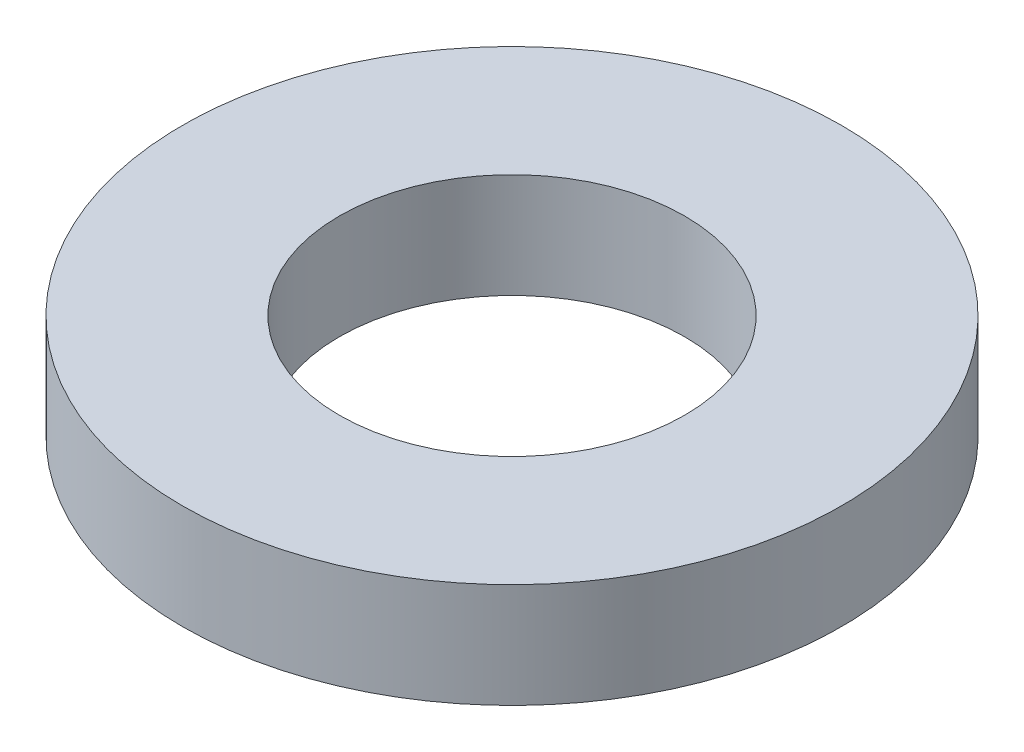
from build123d import *

# Parameters (mm, degrees)
WASHER_PROFILE_63_X_33_R   = 31.5
WASHER_PROFILE_63_X_33_R_2 = 16.5
WASHER_BODY_10MM_DEPTH     = 5


with BuildPart() as part:
    # Washer Profile Ø63 x Ø33 → Washer Body 10mm (new, symmetric)
    with BuildSketch(Plane(origin=(0, 0, 0), x_dir=(1, 0, 0), z_dir=(0, 1, 0))):
        with Locations(Location((0, 0, 0), (0, 0, 270))):
            Circle(WASHER_PROFILE_63_X_33_R)
        with Locations(Location((0, 0, 0), (0, 0, 270))):
            Circle(WASHER_PROFILE_63_X_33_R_2, mode=Mode.SUBTRACT)
    extrude(amount=WASHER_BODY_10MM_DEPTH, both=True)


solid = part.part
